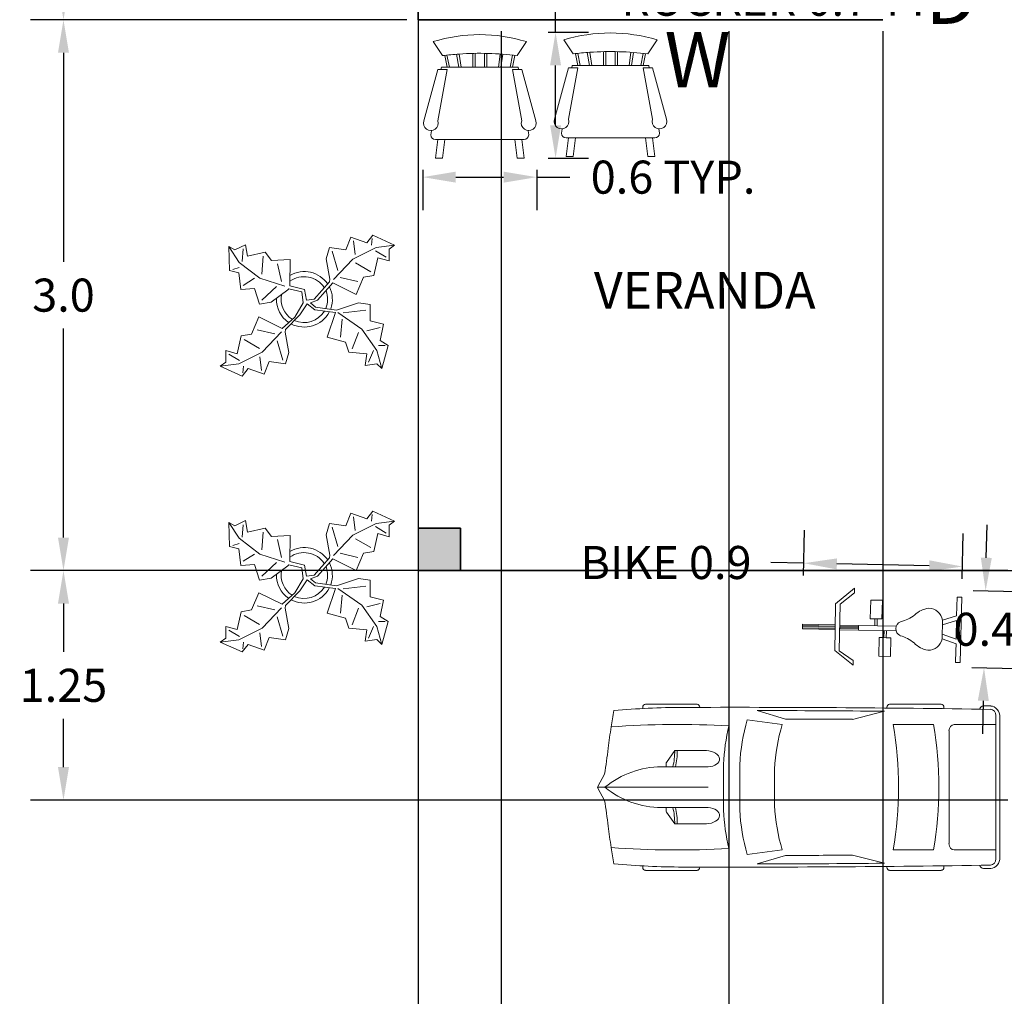
# Model space of a CAD drawing. Units: metres. Extents: x 40.9 to 56.1, y -1.4 to 24.2.
# Tile 2 of 7: x 43.1 to 48.4, y 7.6 to 12.9. Entities that reach past the tile are written whole.
import ezdxf

# ---------------------------------------------------------------- set-up
doc = ezdxf.new("R2010")
doc.units = ezdxf.units.M
doc.header["$MEASUREMENT"] = 0
for name, color, linetype, lineweight in [('A-ANNO-DIMS', 2, 'Continuous', 18), ('A-ANNO-TEXT', 7, 'Continuous', 18), ('A-AREA-IDEN', 7, 'Continuous', 18), ('A-COLS', 7, 'Continuous', 35), ('A-COLS-PATT', 252, 'Continuous', 13), ('A-EQPM', 8, 'Continuous', 18), ('A-FLOR', 7, 'Continuous', 25), ('A-FURN', 8, 'Continuous', 18), ('A-WALL', 7, 'Continuous', 35), ('C-VEHI', 8, 'Continuous', 13), ('L-PLNT', 94, 'Continuous', 13)]:
    doc.layers.add(name, color=color, linetype=linetype, lineweight=lineweight)
doc.styles.get("Standard").update_dxf_attribs({"font": 'arial.ttf'})
doc.dimstyles.get("Standard").update_dxf_attribs({"dimtxt": 0.18, "dimasz": 0.18, "dimexe": 0.18, "dimexo": 0.0625, "dimgap": 0.09, "dimtad": 0, "dimtih": 1, "dimtoh": 1, "dimdec": 1, "dimzin": 0, "dimdsep": 46, "dimtxsty": 'Standard', "dimcen": 0.09, "dimadec": 0, "dimazin": 0, "dimtfac": 1, "dimtdec": 1, "dimtofl": 0, "dimtmove": 0, "dimatfit": 3, "dimfxl": 1, "dimtolj": 1, "dimtzin": 0, "dimarcsym": 0})

# ---------------------------------------------------------------- blocks, each defined once
blk = doc.blocks.new('Chair - Rocking')
for p, q in [((-8, -4.5), (-10, -1.5)), ((8, -4.5), (10, -1.5)), ((-4.5, -7), (-4.96674, -4.19951)), ((-4, -7), (-4.40532, -4.16272)), ((-1.5, -4.05012), (-1.5, -7)), ((-1, -7), (-1, -4.05012)), ((1, -7), (1, -4.04655)), ((1.5, -4.05012), (1.5, -7)), ((4, -7), (4.40187, -4.18694)), ((4.5, -7), (4.96761, -4.19437)), ((-7.5, -4.5), (-7, -7)), ((-6.5, -7), (-7.02225, -4.43)), ((6.5, -7), (7, -4.4057)), ((7.5, -4.5), (7, -7)), ((-9, -7.5), (-12, -18.49999)), ((-7, -7.5), (-9, -7.5)), ((-9, -18.49999), (-7, -7.5)), ((-8.23428, -6.99939), (-8.3093, -7.47958)), ((-8.23041, -7), (8.23915, -7)), ((7, -7.5), (9, -7.5)), ((9, -18.49999), (7, -7.5)), ((8.31071, -7.48854), (8.23449, -7.00073)), ((9, -7.5), (12, -18.49999)), ((-10.36644, -20.64523), (-10.5, -21.49999)), ((10.5, -21.49999), (10.3575, -20.58798)), ((-9, -22.49999), (-9.5, -26.49999)), ((0, -22.49999), (-9.5, -22.49999)), ((-8, -26.49999), (-7.5, -22.49999)), ((0, -22.49999), (9.5, -22.49999)), ((8, -26.49999), (7.5, -22.49999)), ((9, -22.49999), (9.5, -26.49999)), ((-9.5, -26.49999), (-8, -26.49999)), ((9.5, -26.49999), (8, -26.49999))]:
    blk.add_line(p, q)
for centre, radius, start, end in [((0, -34.08333), 34.08333, 72.93847, 107.0615), ((0, -68.25004), 64.25, 93.92211, 97.15267), ((0, -68.25004), 64.25, 82.84733, 93.92211), ((-10.5, -18.99999), 1.58114, 161.5651, 18.43495), ((10.5, -18.99999), 1.58114, 161.5651, 18.43495), ((-9.5, -21.49999), 1, 180, 270), ((9.5, -21.49999), 1, 270, 0)]:
    blk.add_arc(centre, radius, start, end)
blk = doc.blocks.new('*U28')
for p, q in [((536, 950), (536, 936)), ((1182, 988), (568, 988)), ((1214, 950), (1214, 950)), ((3440, 942), (3440, 950)), ((3472, 988), (4087, 988)), ((4119, 950), (4119, 934)), ((2235, 810), (1899, 912)), ((3412, 904), (3030, 807)), ((4736, -851), (4736, 851)), ((4785, -832), (4785, 832)), ((1779, 801), (2195, 746)), ((3516, 746), (3994, 746)), ((4736, 746), (4242, 746)), ((4179, 670), (4179, -670)), ((820, 295), (918, 436)), ((918, 436), (1294, 436)), ((756, 241), (1313, 241)), ((816, 241), (816, 283)), ((1496, -274), (1496, 274)), ((1690, -267), (1690, 267)), ((4736, -267), (4736, 267)), ((83, 156), (3, 10)), ((2102, 216), (2102, -216)), ((0, 0), (1313, 0)), ((3, -10), (83, -156)), ((756, -241), (1313, -241)), ((816, -241), (816, -283)), ((820, -295), (918, -436)), ((918, -436), (1294, -436)), ((2195, -746), (1779, -801)), ((2235, -810), (1899, -912)), ((3412, -904), (3030, -807)), ((3994, -746), (3516, -746)), ((4242, -746), (4736, -746)), ((536, -950), (536, -936)), ((4119, -950), (4119, -934)), ((1182, -988), (568, -988)), ((1214, -950), (1214, -950)), ((3440, -942), (3440, -950)), ((3472, -988), (4087, -988))]:
    blk.add_line(p, q)
for centre, major_axis, ratio, start_param, end_param in [((1046, -12468), (0, 13417), 0.842304, 0.00281, 0.075598), ((568, 950), (0, -37.6), 0.842304, 3.141593, 4.712389), ((1638, -268113), (0, 269063), 0.842304, -0.013397, 0.002797), ((1182, 950), (0, 37.6), 0.842304, -1.570796, 0), ((3472, 950), (0, -37.6), 0.842304, 3.141593, 4.712389), ((4087, 950), (0, 37.6), 0.842304, -1.570796, 0), ((4588, 910), (0, 56.4), 0.842304, -0.013017, 1.249894), ((1638, -268131), (0, 269121), 0.842304, -0.013397, -0.013017), ((4673, 832), (0, -133), 0.842304, 1.570796, 3.128196), ((6757, -699), (0, 7958), 0.842304, 1.367076, 1.39176), ((1638, -268113), (0, -269025), 0.842304, 3.133765, 3.140441), ((4673, 851), (0, -75.2), 0.842304, 1.570796, 3.128196), ((6583, -699), (0, -7755), 0.842304, 4.528606, 4.561838), ((952, -15087), (0, -15833), 0.842304, 3.096046, 3.200911), ((3414, 137), (0, -2280), 0.842304, 4.449482, 4.652344), ((3436, 137), (0, 2077), 0.842304, 1.245306, 1.50788), ((3800, 71), (0, -2021), 0.842304, 4.372215, 4.640744), ((2433, -93125), (0, -93935), 0.842304, 3.134049, 3.144098), ((434, 0), (0, 3734), 0.842304, 4.511394, 4.913384), ((912, 0), (0, 3734), 0.842304, 4.511394, 4.913384), ((4242, 670), (0, 75.2), 0.842304, 0, 1.570796), ((-5194, 1331), (0, -6374), 0.842304, 1.385369, 1.434372), ((331, 432), (0, 696), 0.842304, 4.435146, 4.718221), ((361, 432), (0, 696), 0.842304, 4.435146, 4.718221), ((1290, 339), (161, -9), 0.603834, -1.395552, 1.581315), ((756, -1185), (0, 1427), 0.842304, 0, 0.590319), ((832, 283), (0, 18.8), 0.842304, 0.879714, 1.570796), ((16, 0), (0, -18.8), 0.842304, 4.131459, 5.293319), ((756, 1185), (0, 1427), 0.842304, 2.551274, 3.141593), ((-5194, -1331), (0, 6374), 0.842304, -1.434372, -1.385369), ((3800, -71), (0, -2021), 0.842304, -1.499151, -1.230623), ((832, -283), (0, -18.8), 0.842304, 4.712389, 5.403472), ((331, -432), (0, -696), 0.842304, 1.564964, 1.848039), ((361, -432), (0, -696), 0.842304, 1.564964, 1.848039), ((3414, -137), (0, -2280), 0.842304, -1.510751, -1.307889), ((3436, -137), (0, -2077), 0.842304, -1.50788, -1.245306), ((6583, 699), (0, 7755), 0.842304, 1.721348, 1.754579), ((4242, -670), (0, -75.2), 0.842304, 4.712389, 6.283185), ((6757, 699), (0, 7958), 0.842304, 1.749832, 1.774517), ((952, 15087), (0, -15833), 0.842304, -0.059319, 0.045547), ((2433, 93125), (0, -93935), 0.842304, -0.002505, 0.007544), ((1046, 12468), (0, -13417), 0.842304, -0.075598, -0.00281), ((1638, 268113), (0, 269063), 0.842304, 3.138796, 3.15499), ((1638, 268113), (0, -269025), 0.842304, 0.001152, 0.007828), ((4588, -910), (0, -56.4), 0.842304, -1.249894, 0.013017), ((4673, -851), (0, 75.2), 0.842304, 3.15499, 4.712389), ((4673, -832), (0, -133), 0.842304, 0.013397, 1.570796), ((568, -950), (0, 37.6), 0.842304, 1.570796, 3.141593), ((1182, -950), (0, -37.6), 0.842304, 0, 1.570796), ((3472, -950), (0, -37.6), 0.842304, -1.570796, 0), ((4087, -950), (0, 37.6), 0.842304, 3.141593, 4.712389), ((1638, 268131), (0, 269121), 0.842304, 3.15461, 3.15499)]:
    blk.add_ellipse(centre, major_axis=major_axis, ratio=ratio, start_param=start_param, end_param=end_param)
at = {"extrusion": (0, 0, -1)}
blk.add_ellipse((1290, -339), major_axis=(161, 9), ratio=0.603834, start_param=-1.395552, end_param=1.581315, dxfattribs=at)
blk = doc.blocks.new('Exercise Bike')
for p, q in [((-0.75, 10), (-0.75, 17)), ((-0.75, 17), (0.25, 17)), ((-0.5, 17), (-0.5, 9.9929)), ((-0.25, 10), (-0.25, 17)), ((0, 17), (0, 9.9929)), ((0.25, 17), (0.25, 10)), ((-5.25, 10), (-8.25, 6)), ((-7.25, 6), (-5.25, 9)), ((-0.75, 10), (-5.25, 10)), ((-5.25, 9), (4.75, 9)), ((4.75, 10), (-0.75, 10)), ((-0.75, 5), (-0.75, 9)), ((-0.5, 8.9396), (-0.5, 5)), ((-0.25, 5), (-0.25, 9)), ((0, 8.9396), (0, 5)), ((0.25, 9), (0.25, 5)), ((8.25, 6), (4.75, 10)), ((4.75, 9), (7.25, 6)), ((-8.25, 6), (-7.25, 6)), ((-0.75, -3.0635), (-0.75, 5)), ((-0.75, 5), (0.25, 5)), ((0.25, 5), (0.25, -3.0635)), ((7.25, 6), (8.25, 6)), ((1.75, 2.5), (5.75, 2.5)), ((1.75, 1.5), (1.75, 2.5)), ((5.75, 2.5), (5.75, 0)), ((-6.25, -2), (-6.25, 0.5)), ((-2.25, 0.5), (-6.25, 0.5)), ((-2.25, -0.5), (-2.25, 0.5)), ((0.25, 1.5), (1.75, 1.5)), ((0.25, 1), (1.75, 1)), ((1.75, 1.5), (1.75, 0)), ((1.75, 0), (5.75, 0)), ((-2.25, -2), (-6.25, -2)), ((-2.25, -0.5), (-0.75, -0.5)), ((-2.25, -1), (-2.25, -0.5)), ((-2.25, -1), (-2.25, -2)), ((-0.75, -1), (-2.25, -1)), ((-2.25, -13), (-3.25, -16)), ((-2.25, -16), (-1.25, -13)), ((-2.25, -13), (1.75, -13)), ((0.75, -13), (1.75, -16)), ((1.75, -13), (2.75, -16)), ((-7.25, -16), (-7.25, -17)), ((-4.75, -16), (-7.25, -16)), ((-3.25, -16), (-4.75, -16)), ((1.75, -16), (-2.25, -16)), ((6.75, -16), (2.75, -16)), ((6.75, -17), (6.75, -16)), ((-7.25, -17), (6.75, -17))]:
    blk.add_line(p, q)
for centre, radius, start, end in [((-9.6692, -1.9154), 8.1889, 321.6175, 345.2525), ((-0.25, -4.625), 1.625, 22.61987, 157.3801), ((9.1691, -1.9154), 8.1889, 194.7476, 218.3825), ((0.1685, -10.5843), 4.9531, 133.6443, 173.2256), ((-0.6686, -10.5843), 4.9531, 6.774486, 46.35562), ((-1.7006, -10.0005), 3.0494, 179.9906, 259.6205), ((1.2006, -10.0005), 3.0494, 280.3795, 0.009389)]:
    blk.add_arc(centre, radius, start, end)
blk = doc.blocks.new('Plant - Rubber or Philodendron')
for p, q in [((8.8871, 10.7908), (9.9809, 13.4933)), ((9.9809, 13.4933), (13.3837, 12.301)), ((10.5828, 12.6946), (10.8893, 9.7953)), ((13.3837, 12.301), (14.68, 13.9039)), ((14.5816, 13.2037), (14.3848, 11.8033)), ((14.68, 13.9039), (19.3848, 11.8146)), ((-16.2005, 11.4774), (-13.9899, 8.1064)), ((-16.2005, 11.4774), (-14.8639, 10.7964)), ((-16.0159, 6.3329), (-16.2005, 11.4774)), ((-14.8639, 10.7964), (-12.6195, 11.8975)), ((-13.3174, 8.325), (-13.0735, 11.0065)), ((-12.6195, 11.8975), (-12.1909, 9.4345)), ((4.6914, 8.8812), (5.3859, 11.2828)), ((5.3859, 11.2828), (8.8871, 10.7908)), ((15.3859, 11.3055), (10.3916, 8.7942)), ((15.2875, 10.6053), (17.5907, 9.2105)), ((19.3848, 11.8146), (15.3859, 11.3055)), ((19.3848, 11.8146), (18.1868, 10.9119)), ((18.1868, 10.9119), (18.1925, 8.4119)), ((-12.1909, 9.4345), (-8.3829, 10.3)), ((-8.8369, 9.409), (-9.0894, 5.6095)), ((-8.3829, 10.3), (-7.0549, 8.501)), ((-7.0549, 8.501), (-3.0284, 8.6941)), ((-3.0284, 8.6941), (-3.0709, 3.1041)), ((4.6914, 8.8812), (5.5014, 4.4831)), ((5.9878, 10.4842), (7.1971, 6.3869)), ((10.3916, 8.7942), (6.2847, 4.4028)), ((15.7909, 9.1065), (14.8995, 5.3044)), ((18.1925, 8.4119), (15.7909, 9.1065)), ((-15.3434, 6.5514), (-13.9984, 6.9884)), ((-13.9899, 8.1064), (-9.5434, 4.7185)), ((-4.8529, 4.012), (-5.7184, 7.82)), ((14.2977, 6.1031), (10.9934, 7.9956)), ((-14.0069, 5.8704), (-16.0159, 6.3329)), ((-13.5868, 2.2894), (-14.0069, 5.8704)), ((-13.1329, 3.1804), (-10.6614, 4.727)), ((-9.5434, 4.7185), (-4.1917, 2.9888)), ((5.4346, 3.9146), (5.5014, 4.4831)), ((7.7005, 4.8881), (11.5025, 3.9967)), ((12.7005, 4.8994), (11.1089, 1.1958)), ((14.8995, 5.3044), (12.7005, 4.8994)), ((-10.6784, 2.491), (-13.5868, 2.2894)), ((-9.5858, -0.8715), (-10.6784, 2.491)), ((-9.1318, 0.0195), (-5.9793, 2.9025)), ((-7.1228, -0.443), (-3.5248, 2.2131)), ((-3.5248, 2.2131), (-3.3011, 2.4355)), ((-3.3011, 2.4355), (-0.5306, 1.7947)), ((-3.0709, 3.1041), (0.0797, 2.3163)), ((0.0797, 2.3163), (0.4866, -0.031)), ((2.1141, 0.2298), (5.4346, 3.9146)), ((6.1032, 3.6844), (2.8262, -0.031)), ((11.1089, 1.1958), (6.1032, 3.6844)), ((-0.5306, 1.7947), (-0.2255, -0.5527)), ((-0.5306, 1.7947), (-0.5306, 1.7947)), ((0.4866, -0.031), (2.1141, 0.2298)), ((-7.1228, -0.443), (-9.5858, -0.8715)), ((-2.019, -3.6148), (-0.2255, -0.5527)), ((-0.9375, -3.1608), (0.5883, -0.8135)), ((0.5883, -0.8135), (2.2447, -2.0916)), ((2.8262, -0.031), (1.3003, -0.5527)), ((1.3003, -0.5527), (2.4193, -1.4655)), ((2.2447, -2.0916), (6.7108, -2.6626)), ((2.4193, -1.4655), (6.895, -2.1175)), ((11.6605, -0.5413), (6.895, -2.1175)), ((11.6605, -0.5413), (14.1354, -0.8948)), ((14.1354, -0.8948), (14.1354, -4.4304)), ((-11.3237, -7.2629), (-9.7321, -3.5593)), ((-9.7321, -3.5593), (-4.7264, -6.0479)), ((-2.019, -3.6148), (-4.7264, -6.0479)), ((-4.0579, -6.2781), (-0.9375, -3.1608)), ((4.943, -7.9659), (6.7108, -2.6626)), ((12.3677, -6.1981), (7.219, -2.6772)), ((8.125, -4.0768), (7.7715, -7.9659)), ((8.3544, -2.7453), (13.1973, -2.1704)), ((-4.1246, -6.8466), (-4.0579, -6.2781)), ((15.5496, -10.7943), (12.3677, -6.1981)), ((16.2567, -5.8446), (13.4283, -6.5517)), ((14.1354, -4.4304), (16.9638, -5.1375)), ((16.9638, -5.1375), (16.2567, -8.673)), ((-14.4141, -11.4699), (-13.5228, -7.6679)), ((-13.5228, -7.6679), (-11.3237, -7.2629)), ((-6.3237, -7.2516), (-10.1257, -6.3602)), ((-9.0148, -11.1577), (-4.9047, -6.8122)), ((-3.3146, -11.2447), (-4.1246, -6.8466)), ((8.8321, -9.0266), (4.943, -7.9659)), ((10.2463, -10.4408), (11.6605, -6.9053)), ((-12.921, -8.4665), (-9.6166, -10.359)), ((-4.611, -12.8477), (-5.8203, -8.7504)), ((9.5392, -11.1479), (8.8321, -9.0266)), ((17.3174, -9.7337), (15.9032, -9.7337)), ((16.2567, -8.673), (18.0245, -9.7337)), ((18.0245, -9.7337), (16.6103, -14.6834)), ((-16.8157, -10.7754), (-14.4141, -11.4699)), ((-16.8101, -13.2754), (-16.8157, -10.7754)), ((-13.9107, -12.9688), (-16.2139, -11.574)), ((-14.0091, -13.669), (-9.0148, -11.1577)), ((-9.206, -15.0581), (-9.5126, -12.1588)), ((-3.3146, -11.2447), (-4.0092, -13.6463)), ((13.4283, -11.5015), (9.5392, -11.1479)), ((13.0748, -13.9763), (13.4283, -11.5015)), ((14.8425, -10.7943), (13.7819, -13.2692)), ((16.6103, -14.6834), (15.5496, -10.7943)), ((-18.008, -14.1781), (-16.8101, -13.2754)), ((-18.008, -14.1781), (-14.0091, -13.669)), ((-13.3032, -16.2674), (-18.008, -14.1781)), ((-12.0069, -14.6645), (-13.3032, -16.2674)), ((-13.2048, -15.5672), (-13.008, -14.1668)), ((-8.6042, -15.8568), (-12.0069, -14.6645)), ((-7.5103, -13.1543), (-8.6042, -15.8568)), ((-4.0092, -13.6463), (-7.5103, -13.1543)), ((15.5496, -13.6228), (13.0748, -13.9763)), ((16.6103, -14.6834), (15.5496, -13.6228))]:
    blk.add_line(p, q)
for centre, radius, start, end in [((0, 0), 6.1275, 34.37569, 120.1028), ((-0.0601, -0.2075), 5.2461, 33.82192, 124.9414), ((-0.098, 0.1364), 6.1288, 341.2017, 26.09184), ((0.0308, 0.1664), 6, 178.6147, 235.1169), ((0.0308, 0.1664), 5, 168.1647, 238.6725), ((-0.2664, 0.1682), 5.2775, 338.4094, 20.03007), ((-0.0234, 0.3825), 6.1492, 242.5812, 331.2714), ((-0.1102, 0.4886), 5.2883, 247.3711, 327.472)]:
    blk.add_arc(centre, radius, start, end)
blk = doc.blocks.new('*D87')
at = {"layer": 'A-ANNO-DIMS', "color": 0, "lineweight": -2, "transparency": 16777216}
for p, q in [((46.0031, 12.8585), (46.0031, 13.0385)), ((46.0031, 13.0385), (46.1831, 13.0385)), ((45.9627, 12.8585), (46.1831, 12.8585)), ((46.0031, 12.3527), (46.0031, 12.6785)), ((45.9627, 12.1727), (46.1831, 12.1727))]:
    blk.add_line(p, q, dxfattribs=at)
at = {"layer": 'A-ANNO-DIMS', "color": 0, "transparency": 16777216}
for points in [[(45.9731, 12.6785), (46.0331, 12.6785), (46.0031, 12.8585)], [(45.9731, 12.3527), (46.0331, 12.3527), (46.0031, 12.1727)]]:
    blk.add_solid(points, dxfattribs=at)
at = {"layer": 'Defpoints', "color": 0, "transparency": 16777216}
for p in [(45.9002, 12.8585), (46.0031, 12.8585), (45.9002, 12.1727)]:
    blk.add_point(p, dxfattribs=at)
at = {"layer": 'A-ANNO-DIMS', "color": 0, "transparency": 16777216, "insert": (47.3143, 13.0385), "char_height": 0.18, "attachment_point": 5}
blk.add_mtext('\\A1;ROCKER 0.7 TYP.', dxfattribs=at)
blk = doc.blocks.new('*D88')
at = {"layer": 'A-ANNO-DIMS', "color": 0, "lineweight": -2, "transparency": 16777216}
for p, q in [((45.2796, 12.1102), (45.2796, 11.8898)), ((45.4596, 12.0698), (45.7202, 12.0698)), ((45.9002, 12.1102), (45.9002, 11.8898)), ((45.9002, 12.0698), (46.0802, 12.0698))]:
    blk.add_line(p, q, dxfattribs=at)
at = {"layer": 'A-ANNO-DIMS', "color": 0, "transparency": 16777216}
for points in [[(45.4596, 12.0998), (45.4596, 12.0398), (45.2796, 12.0698)], [(45.7202, 12.0998), (45.7202, 12.0398), (45.9002, 12.0698)]]:
    blk.add_solid(points, dxfattribs=at)
at = {"layer": 'Defpoints', "color": 0, "transparency": 16777216}
for p in [(45.2796, 12.1727), (45.9002, 12.1727), (45.9002, 12.0698)]:
    blk.add_point(p, dxfattribs=at)
at = {"layer": 'A-ANNO-DIMS', "color": 0, "transparency": 16777216, "insert": (46.6432, 12.0698), "char_height": 0.18, "attachment_point": 5}
blk.add_mtext('\\A1;0.6 TYP.', dxfattribs=at)
blk = doc.blocks.new('*D113')
at = {"layer": 'A-ANNO-DIMS', "color": 0, "lineweight": -2, "transparency": 16777216}
for p, q in [((47.3544, 9.9003), (47.3596, 10.1473)), ((48.2178, 9.8823), (48.223, 10.1293)), ((47.3558, 9.9674), (47.1758, 9.9711)), ((48.0393, 9.9531), (47.5358, 9.9636))]:
    blk.add_line(p, q, dxfattribs=at)
at = {"layer": 'A-ANNO-DIMS', "color": 0, "transparency": 16777216}
for points in [[(47.5364, 9.9936), (47.5351, 9.9336), (47.3558, 9.9674)], [(48.0399, 9.9831), (48.0386, 9.9231), (48.2192, 9.9493)]]:
    blk.add_solid(points, dxfattribs=at)
at = {"layer": 'Defpoints', "color": 0, "transparency": 16777216}
for p in [(47.3558, 9.9674), (47.3531, 9.8378), (48.2165, 9.8198)]:
    blk.add_point(p, dxfattribs=at)
at = {"layer": 'A-ANNO-DIMS', "color": 0, "transparency": 16777216, "insert": (46.6044, 9.9711), "char_height": 0.18, "attachment_point": 5}
blk.add_mtext('\\A1;BIKE 0.9', dxfattribs=at)
blk = doc.blocks.new('*D114')
at = {"layer": 'A-ANNO-DIMS', "color": 0, "lineweight": -2, "transparency": 16777216}
for p, q in [((48.3498, 9.997), (48.3536, 10.177)), ((48.279, 9.8185), (48.526, 9.8133)), ((48.2702, 9.3995), (48.5172, 9.3943)), ((48.3335, 9.2181), (48.3297, 9.0381))]:
    blk.add_line(p, q, dxfattribs=at)
at = {"layer": 'A-ANNO-DIMS', "color": 0, "transparency": 16777216}
for points in [[(48.3198, 9.9977), (48.3798, 9.9964), (48.346, 9.8171)], [(48.3035, 9.2187), (48.3635, 9.2175), (48.3373, 9.3981)]]:
    blk.add_solid(points, dxfattribs=at)
at = {"layer": 'Defpoints', "color": 0, "transparency": 16777216}
for p in [(48.2165, 9.8198), (48.346, 9.8171), (48.2077, 9.4008)]:
    blk.add_point(p, dxfattribs=at)
at = {"layer": 'A-ANNO-DIMS', "color": 0, "transparency": 16777216, "insert": (48.3416, 9.6076), "char_height": 0.18, "attachment_point": 5}
blk.add_mtext('\\A1;0.4', dxfattribs=at)
blk = doc.blocks.new('*D130')
at = {"layer": 'A-ANNO-DIMS', "color": 0, "lineweight": -2, "transparency": 16777216}
for p, q in [((45.1927, 12.9273), (43.1421, 12.9273)), ((43.3221, 12.7473), (43.3221, 11.6092)), ((43.3221, 10.1073), (43.3221, 11.2453)), ((45.1927, 9.9273), (43.1421, 9.9273))]:
    blk.add_line(p, q, dxfattribs=at)
at = {"layer": 'A-ANNO-DIMS', "color": 0, "transparency": 16777216}
for points in [[(43.2921, 12.7473), (43.3521, 12.7473), (43.3221, 12.9273)], [(43.2921, 10.1073), (43.3521, 10.1073), (43.3221, 9.9273)]]:
    blk.add_solid(points, dxfattribs=at)
at = {"layer": 'Defpoints', "color": 0, "transparency": 16777216}
for p in [(43.3221, 12.9273), (45.2552, 12.9273), (45.2552, 9.9273)]:
    blk.add_point(p, dxfattribs=at)
at = {"layer": 'A-ANNO-DIMS', "color": 0, "transparency": 16777216, "insert": (43.3221, 11.4273), "char_height": 0.18, "attachment_point": 5}
blk.add_mtext('\\A1;3.0', dxfattribs=at)
blk = doc.blocks.new('*D131')
at = {"layer": 'A-ANNO-DIMS', "color": 0, "lineweight": -2, "transparency": 16777216}
for p, q in [((48.4677, 9.9273), (43.1421, 9.9273)), ((43.3221, 9.7473), (43.3221, 9.4842)), ((43.3221, 8.8573), (43.3221, 9.1203)), ((48.4677, 8.6773), (43.1421, 8.6773))]:
    blk.add_line(p, q, dxfattribs=at)
at = {"layer": 'A-ANNO-DIMS', "color": 0, "transparency": 16777216}
for points in [[(43.2921, 9.7473), (43.3521, 9.7473), (43.3221, 9.9273)], [(43.2921, 8.8573), (43.3521, 8.8573), (43.3221, 8.6773)]]:
    blk.add_solid(points, dxfattribs=at)
at = {"layer": 'Defpoints', "color": 0, "transparency": 16777216}
for p in [(43.3221, 9.9273), (48.5302, 9.9273), (48.5302, 8.6773)]:
    blk.add_point(p, dxfattribs=at)
at = {"layer": 'A-ANNO-DIMS', "color": 0, "transparency": 16777216, "insert": (43.3221, 9.3023), "char_height": 0.18, "attachment_point": 5}
blk.add_mtext('\\A1;1.25', dxfattribs=at)
blk = doc.blocks.new('*D137')
at = {"layer": 'A-ANNO-DIMS', "color": 0, "lineweight": -2, "transparency": 16777216}
for p, q in [((43.3221, 13.7723), (43.3221, 13.9523)), ((43.3221, 13.9523), (43.5021, 13.9523)), ((45.1927, 13.7723), (43.1421, 13.7723)), ((43.3221, 13.1073), (43.3221, 13.5923)), ((45.1927, 12.9273), (43.1421, 12.9273))]:
    blk.add_line(p, q, dxfattribs=at)
at = {"layer": 'A-ANNO-DIMS', "color": 0, "transparency": 16777216}
for points in [[(43.2921, 13.5923), (43.3521, 13.5923), (43.3221, 13.7723)], [(43.2921, 13.1073), (43.3521, 13.1073), (43.3221, 12.9273)]]:
    blk.add_solid(points, dxfattribs=at)
at = {"layer": 'Defpoints', "color": 0, "transparency": 16777216}
for p in [(43.3221, 13.7723), (45.2552, 13.7723), (45.2552, 12.9273)]:
    blk.add_point(p, dxfattribs=at)
at = {"layer": 'A-ANNO-DIMS', "color": 0, "transparency": 16777216, "insert": (43.8965, 13.9523), "char_height": 0.18, "attachment_point": 5}
blk.add_mtext('\\A1;0.845', dxfattribs=at)
blk = doc.blocks.new('*D149')
at = {"layer": 'A-ANNO-DIMS', "color": 0, "lineweight": -2, "transparency": 16777216}
for p, q in [((45.2552, 12.8648), (45.2552, 6.6791)), ((45.7075, 12.8648), (45.7075, 6.6791)), ((45.0752, 6.8591), (44.8952, 6.8591)), ((45.8875, 6.8591), (46.0675, 6.8591))]:
    blk.add_line(p, q, dxfattribs=at)
at = {"layer": 'A-ANNO-DIMS', "color": 0, "transparency": 16777216}
for points in [[(45.0752, 6.8891), (45.0752, 6.8291), (45.2552, 6.8591)], [(45.8875, 6.8891), (45.8875, 6.8291), (45.7075, 6.8591)]]:
    blk.add_solid(points, dxfattribs=at)
at = {"layer": 'Defpoints', "color": 0, "transparency": 16777216}
for p in [(45.2552, 12.9273), (45.7075, 12.9273), (45.7075, 6.8591)]:
    blk.add_point(p, dxfattribs=at)
at = {"layer": 'A-ANNO-DIMS', "color": 0, "transparency": 16777216, "insert": (46.392, 6.8591), "char_height": 0.18, "attachment_point": 5}
blk.add_mtext('\\A1;0.45', dxfattribs=at)
blk = doc.blocks.new('*D155')
at = {"layer": 'A-ANNO-DIMS', "color": 0, "lineweight": -2, "transparency": 16777216}
for p, q in [((46.947505, 12.864753), (46.947505, 6.679084)), ((47.786899, 12.864753), (47.786899, 6.679084)), ((46.767505, 6.859084), (46.587505, 6.859084)), ((47.966899, 6.859084), (48.146899, 6.859084))]:
    blk.add_line(p, q, dxfattribs=at)
at = {"layer": 'A-ANNO-DIMS', "color": 0, "transparency": 16777216}
for points in [[(46.767505, 6.889084), (46.767505, 6.829084), (46.947505, 6.859084)], [(47.966899, 6.889084), (47.966899, 6.829084), (47.786899, 6.859084)]]:
    blk.add_solid(points, dxfattribs=at)
at = {"layer": 'Defpoints', "color": 0, "transparency": 16777216}
for p in [(46.947505, 12.927253), (47.786899, 12.927253), (47.786899, 6.859084)]:
    blk.add_point(p, dxfattribs=at)
at = {"layer": 'A-ANNO-DIMS', "color": 0, "transparency": 16777216, "insert": (47.367202, 6.859084), "char_height": 0.18, "attachment_point": 5}
blk.add_mtext('\\A1;0.84', dxfattribs=at)
blk = doc.blocks.new('*D156')
at = {"layer": 'A-ANNO-DIMS', "color": 0, "lineweight": -2, "transparency": 16777216}
for p, q in [((47.786899, 12.864753), (47.786899, 6.679084)), ((48.530203, 12.864753), (48.530203, 6.679084)), ((47.606899, 6.859084), (47.426899, 6.859084)), ((48.710203, 6.859084), (48.890203, 6.859084))]:
    blk.add_line(p, q, dxfattribs=at)
at = {"layer": 'A-ANNO-DIMS', "color": 0, "transparency": 16777216}
for points in [[(47.606899, 6.889084), (47.606899, 6.829084), (47.786899, 6.859084)], [(48.710203, 6.889084), (48.710203, 6.829084), (48.530203, 6.859084)]]:
    blk.add_solid(points, dxfattribs=at)
at = {"layer": 'Defpoints', "color": 0, "transparency": 16777216}
for p in [(47.786899, 12.927253), (48.530203, 12.927253), (48.530203, 6.859084)]:
    blk.add_point(p, dxfattribs=at)
at = {"layer": 'A-ANNO-DIMS', "color": 0, "transparency": 16777216, "insert": (48.158551, 6.859084), "char_height": 0.18, "attachment_point": 5}
blk.add_mtext('\\A1;0.74', dxfattribs=at)

msp = doc.modelspace()

# ---------------------------------------------------------------- hatches: boundary and pattern name
at = {"layer": 'A-COLS-PATT'}
h = msp.add_hatch(color=256, dxfattribs=at)
h.dxf.hatch_style = 1
h.paths.add_polyline_path([(45.4852, 10.1573), (45.2552, 10.1573), (45.2552, 9.9273), (45.4852, 9.9273)])

# ---------------------------------------------------------------- linework, layer by layer
at = {"layer": 'A-COLS'}
for p, q in [((45.4852, 10.1573), (45.2552, 10.1573)), ((45.4852, 9.9273), (45.4852, 10.1573)), ((45.2552, 9.9273), (45.4852, 9.9273))]:
    msp.add_line(p, q, dxfattribs=at)
at = {"layer": 'A-FLOR'}
for p, q in [((45.2552, 12.9273), (45.2552, 9.9273)), ((45.2552, 9.9273), (48.5302, 9.9273))]:
    msp.add_line(p, q, dxfattribs=at)
at = {"layer": 'A-WALL'}
for p, q in [((45.2552, 19.8573), (45.2552, 12.9273)), ((45.2552, 12.9273), (47.7869, 12.9273))]:
    msp.add_line(p, q, dxfattribs=at)

# ---------------------------------------------------------------- block references
at = {"layer": 'A-EQPM', "xscale": 0.0254, "yscale": 0.0254, "zscale": 0.0254, "rotation": 88.80109357694278}
msp.add_blockref('Exercise Bike', (47.7804, 9.6193), dxfattribs=at)
at = {"layer": 'A-FURN', "xscale": 0.0254, "yscale": 0.0254, "zscale": 0.0254}
for p in [(45.5899, 12.8458), (46.302, 12.8552)]:
    msp.add_blockref('Chair - Rocking', p, dxfattribs=at)
at = {"layer": 'C-VEHI', "xscale": 0.0004580947929124, "yscale": 0.0004580947929124, "zscale": 0.0004580947929124}
msp.add_blockref('*U28', (46.2322, 8.7473), dxfattribs=at)
at = {"layer": 'L-PLNT', "xscale": 0.0254, "yscale": 0.0254, "zscale": 0.0254}
for p in [(44.634, 11.3998), (44.634, 9.897)]:
    msp.add_blockref('Plant - Rubber or Philodendron', p, dxfattribs=at)

# ---------------------------------------------------------------- texts
at = {"layer": 'A-ANNO-TEXT'}
for s, p in [('D ', (48.0178, 12.9043)), ('W', (46.5969, 12.5597))]:
    msp.add_text(s, height=0.3, dxfattribs=at).set_placement(p)
at = {"layer": 'A-AREA-IDEN', "insert": (46.2119, 11.5541), "char_height": 0.2, "attachment_point": 1}
msp.add_mtext_dynamic_manual_height_columns('VERANDA', width=2.030673, gutter_width=1, heights=[0], dxfattribs=at)

# ---------------------------------------------------------------- dimensions: what is measured, and where the dimension line sits
at = {"layer": 'A-ANNO-DIMS'}
for base, p1, p2, angle, override, picture, middle in [((43.3221, 13.7723), (45.2552, 12.9273), (45.2552, 13.7723), 90, {"dimdec": 3, "dimlfac": 1, "dimrnd": 0, "dimzin": 0, "dimdsep": 46, "dimlunit": 2}, '*D137', (43.8965, 13.9523)), ((43.3221, 12.9273), (45.2552, 9.9273), (45.2552, 12.9273), 90, {"dimdec": 1, "dimlfac": 1, "dimrnd": 0, "dimzin": 0, "dimdsep": 46, "dimlunit": 2}, '*D130', (43.3221, 11.4273)), ((48.346, 9.8171), (48.2077, 9.4008), (48.2165, 9.8198), 88.8011, {"dimdec": 1, "dimlfac": 1, "dimrnd": 0, "dimzin": 0, "dimdsep": 46, "dimlunit": 2}, '*D114', (48.3416, 9.6076)), ((43.3221, 9.9273), (48.5302, 8.6773), (48.5302, 9.9273), 90, {"dimdec": 2, "dimlfac": 1, "dimrnd": 0, "dimzin": 0, "dimdsep": 46, "dimlunit": 2}, '*D131', (43.3221, 9.3023))]:
    dim = msp.add_linear_dim(base=base, p1=p1, p2=p2, angle=angle, dimstyle='Standard', override=override, dxfattribs=at)
    dim.commit()
    dim.dimension.update_dxf_attribs({"geometry": picture, "text_midpoint": middle})
for base, p1, p2, angle, text, picture, middle in [((46.0031, 12.8585), (45.9002, 12.1727), (45.9002, 12.8585), 90, 'ROCKER <> TYP.', '*D87', (47.3143, 13.0385)), ((47.3558, 9.9674), (48.2165, 9.8198), (47.3531, 9.8378), 178.8011, 'BIKE <>', '*D113', (46.6044, 9.9711))]:
    dim = msp.add_linear_dim(base=base, p1=p1, p2=p2, angle=angle, text=text, dimstyle='Standard', override={"dimdec": 1, "dimlfac": 1, "dimrnd": 0, "dimzin": 0, "dimdsep": 46, "dimlunit": 2}, dxfattribs=at)
    dim.commit()
    dim.dimension.update_dxf_attribs({"geometry": picture, "text_midpoint": middle})
for base, p1, p2, picture, middle in [((45.7075, 6.8591), (45.2552, 12.9273), (45.7075, 12.9273), '*D149', (46.392, 6.8591)), ((47.7869, 6.8591), (46.9475, 12.9273), (47.7869, 12.9273), '*D155', (47.3672, 6.8591)), ((48.5302, 6.8591), (47.7869, 12.9273), (48.5302, 12.9273), '*D156', (48.1586, 6.8591))]:
    dim = msp.add_linear_dim(base=base, p1=p1, p2=p2, dimstyle='Standard', override={"dimdec": 2, "dimlfac": 1, "dimrnd": 0, "dimzin": 0, "dimdsep": 46, "dimlunit": 2}, dxfattribs=at)
    dim.commit()
    dim.dimension.update_dxf_attribs({"geometry": picture, "text_midpoint": middle})
dim = msp.add_linear_dim(base=(45.9002, 12.0698), p1=(45.2796, 12.1727), p2=(45.9002, 12.1727), text='<> TYP.', dimstyle='Standard', override={"dimdec": 1, "dimlfac": 1, "dimrnd": 0, "dimzin": 0, "dimdsep": 46, "dimlunit": 2}, dxfattribs=at)
dim.commit()
dim.dimension.update_dxf_attribs({"geometry": '*D88', "text_midpoint": (46.6432, 12.0698)})

doc.saveas('drawing.dxf')
